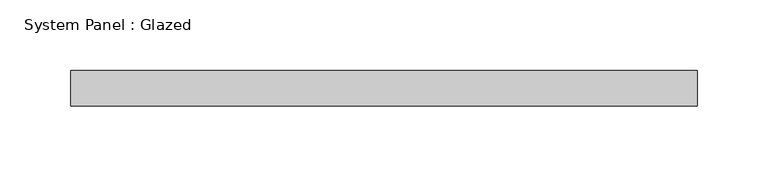
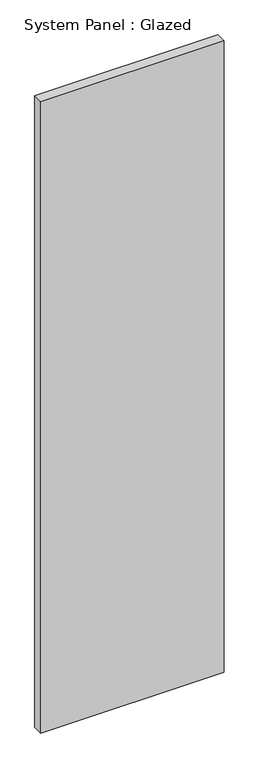
"""IFC4 building model written with IfcOpenShell, lengths in millimetres: plate geometry, System Panel : Glazed."""

from ifc_helpers import new_model, si_unit, origin, origin_with_axes, place, context, project, spatial, polyline, outline, extrude, source, transform, mapped, element, save


def system_panel_glazed_49c4d9bd(model_context):
    return source(origin(), model_context, "Body", "SweptSolid", [
        extrude(outline(polyline([(222.25, 19.05), (-222.25, 19.05), (-222.25, 44.45), (222.25, 44.45), (222.25, 19.05)])), origin_with_axes(), (0.0, 0.0, 1.0), 1618.718644),
    ])


if __name__ == "__main__":
    model = new_model("IFC4")
    model_context = context("Model", 3, world=origin())
    ifc_project = project(units=[si_unit("LENGTHUNIT", "METRE", prefix="MILLI")], contexts=[model_context])
    site = spatial("IfcSite", under=ifc_project)
    building = spatial("IfcBuilding", under=site)
    placement = place(None, origin())
    system_panel_glazed_shape = system_panel_glazed_49c4d9bd(model_context)
    element("IfcPlate", 1, ObjectType="System Panel : Glazed", at=placement, inside=building, context=model_context, shape_type="MappedRepresentation", body=[
        mapped(system_panel_glazed_shape, transform((0.0, 0.0, 0.0), x_axis=(1.0, 0.0, 0.0), y_axis=(0.0, 1.0, 0.0), z_axis=(0.0, 0.0, 1.0))),
    ])
    save(model, "model.ifc")

# Revit data of these elements
# Type "System Panel : Glazed"
#   Construction Type Id = "GSP4R"
#   Analytic Construction = "1/8 in Pilkington single glazing"
#   Visual Light Transmittance = 0.9
#   Solar Heat Gain Coefficient = 0.86
#   Heat Transfer Coefficient (U) = 1.18115 BTU/(h·ft²·°F)
#   Define Thermal Properties by = 1
# Element 1 (IfcPlate, "System Panel : Glazed")
#   Materials on its faces: "Glass"
# Materials
#   "Glass": class "Glass", colour RGB 0 128 192, transparency 0.75, Description = "Soda Lime Glass", Cost = 0
